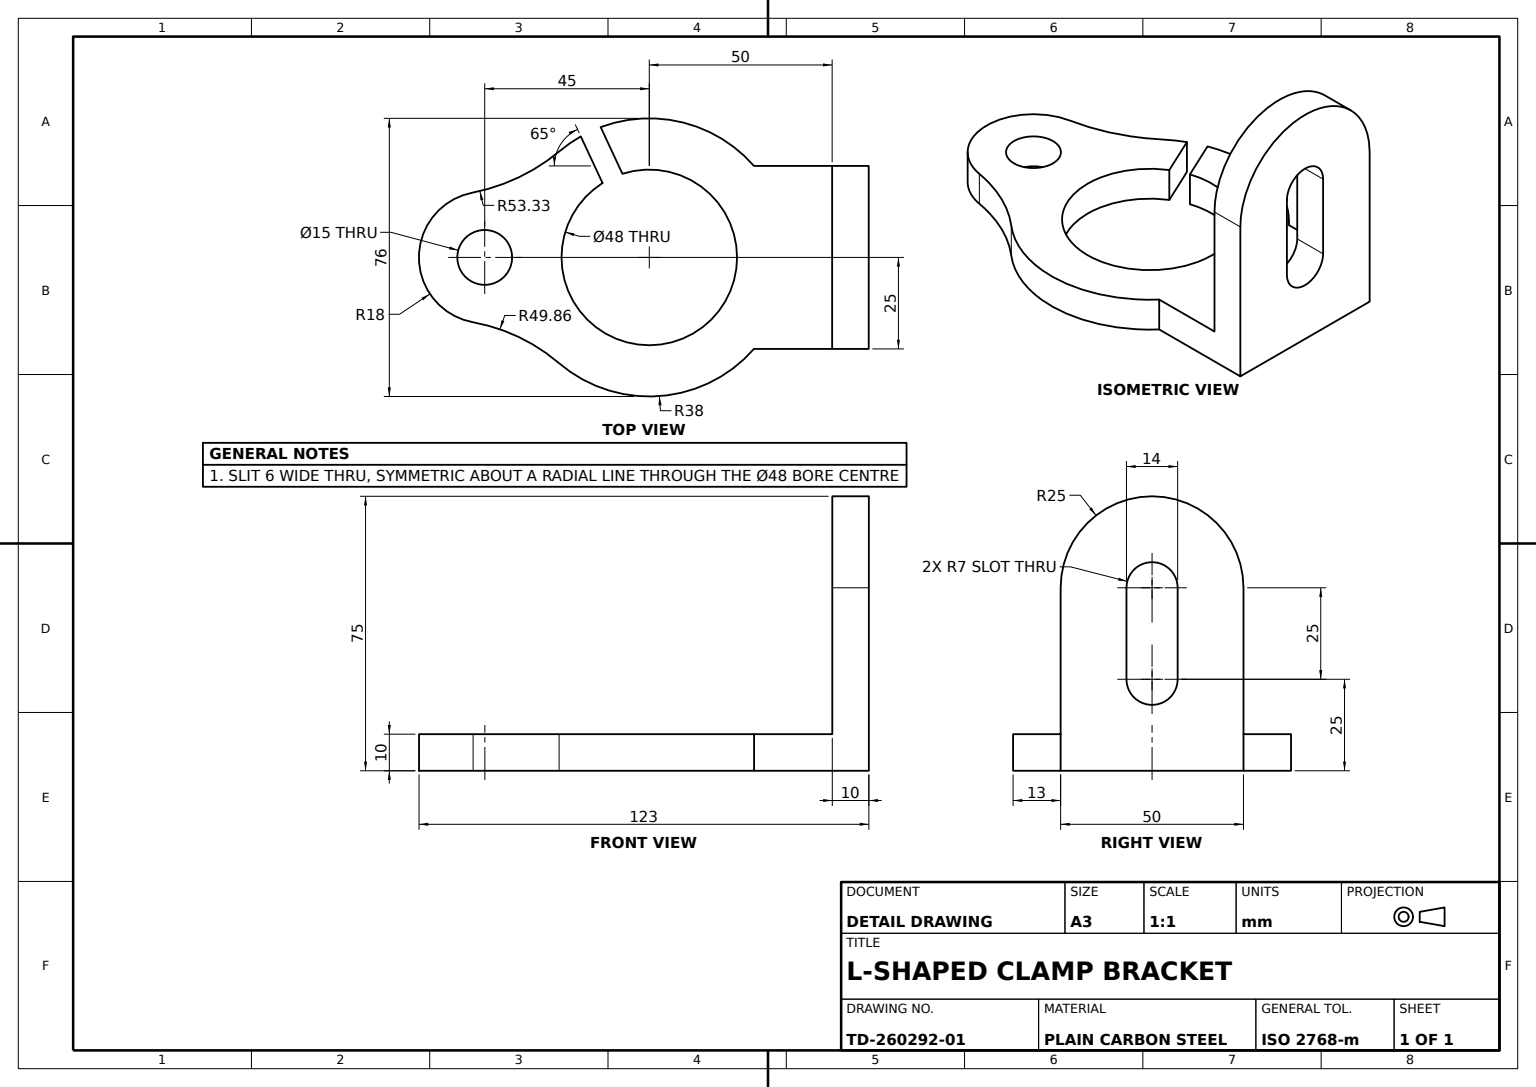
SolidWorks part; units mm, degrees
material "Plain Carbon Steel"
ref_plane "Front Plane" through (0, 0, 0) normal (0, 0, 1) x (1, 0, 0)
ref_plane "Top Plane" through (0, 0, 0) normal (0, 1, 0) x (1, 0, 0)
ref_plane "Right Plane" through (0, 0, 0) normal (1, 0, 0) x (0, 0, -1)
sketch "Clamp Base Profile Sketch" plane through (0, 0, 0) normal (0, 1, 0) x (1, 0, 0)
  line L0 (0, 151.6276) -> (0, -148.3724) construction
  line L7 (0, -61.7492) -> (-40.2239, -80.506) construction
  line L8 (0, -61.7492) -> (-47.1583, -61.7492) construction
  line L10 (-22.8486, -69.0936) -> (-35.6001, -75.0397)
  line L11 (-20.3129, -74.5315) -> (-33.0643, -80.4775)
  line L13 (25, -11.7492) -> (-25, -11.7492)
  line L15 (-25, -33.1311) -> (-25, -11.7492)
  line L17 (25, -33.1311) -> (25, -11.7492)
  arc A3 (-33.0643, -80.4775) -> (-29.1303, -86.1506) centre (0, -61.7492) ccw
  arc A4 (-20.3129, -74.5315) -> (-22.8486, -69.0936) centre (0, -61.7492) ccw
  circle A5 centre (0, -106.7492) radius 7.5
  arc A6 (-17.6675, -110.193) -> (17.7113, -109.9602) centre (0, -106.7492) ccw
  arc A8 (28.8795, -86.4469) -> (17.7113, -109.9602) centre (66.7753, -118.8554) ccw
  arc A9 (-17.6675, -110.193) -> (-29.1303, -86.1506) centre (-70.0124, -120.3959) ccw
  arc A10 (-2.473, -99.6687) -> (2.473, -99.6687) centre (0, -61.7492) ccw
  arc A11 (28.8795, -86.4469) -> (25, -33.1311) centre (0, -61.7492) ccw
  arc A12 (-25, -33.1311) -> (-35.6001, -75.0397) centre (0, -61.7492) ccw
  point P5 (0, -11.7492)
  dimension "D2" = 48
  dimension "D3" = 76
  dimension "D4" = 25
  dimension "D6" = 15
  dimension "D7" = 36
  dimension "D8" = 45
  dimension "D15" = 53.33
  dimension "D16" = 49.8639
  dimension "D1" = 300
  dimension "D5" = 6
  dimension "D9" = 50
  dimension "D10" = 61.7492
  dimension "D11" = 151.6276
  dimension "D12" = 50
  dimension "D13" = 44.3822
  dimension "D14" = 47.1583
extrude "Clamp Base Plate" add sketch "Clamp Base Profile Sketch" along normal mid plane 10 contours L15 A12 L10 A4 L11 A3 A9 A6 A8 A11 L17 L13 A5
sketch "Slotted Tab Profile Sketch" plane through (0, 0, 11.7492) normal (0, 0, -1) x (-1, 0, 0)
  line L0 (0, -5) -> (0, 45) construction
  line L1 (-25, -5) -> (25, -5) construction
  line L2 (-25, -5) -> (-25, 45)
  line L3 (25, -5) -> (25, 45)
  line L4 (0, 45) -> (0, 20) construction
  line L9 (7, 45) -> (7, 20)
  line L10 (-7, 45) -> (-7, 20)
  line L11 (-25, -5) -> (25, -5)
  arc A1 (25, 45) -> (-25, 45) centre (0, 45) ccw
  arc A6 (7, 45) -> (-7, 45) centre (0, 45) ccw
  arc A7 (-7, 20) -> (7, 20) centre (0, 20) ccw
  point P5 (0, 20)
  point P12 (0, 32.5)
  dimension "D1" = 25
  dimension "D4" = 7
  dimension "D2" = 50
  dimension "D3" = 25
extrude "Slotted Upright Tab" add sketch "Slotted Tab Profile Sketch" along normal blind 10
